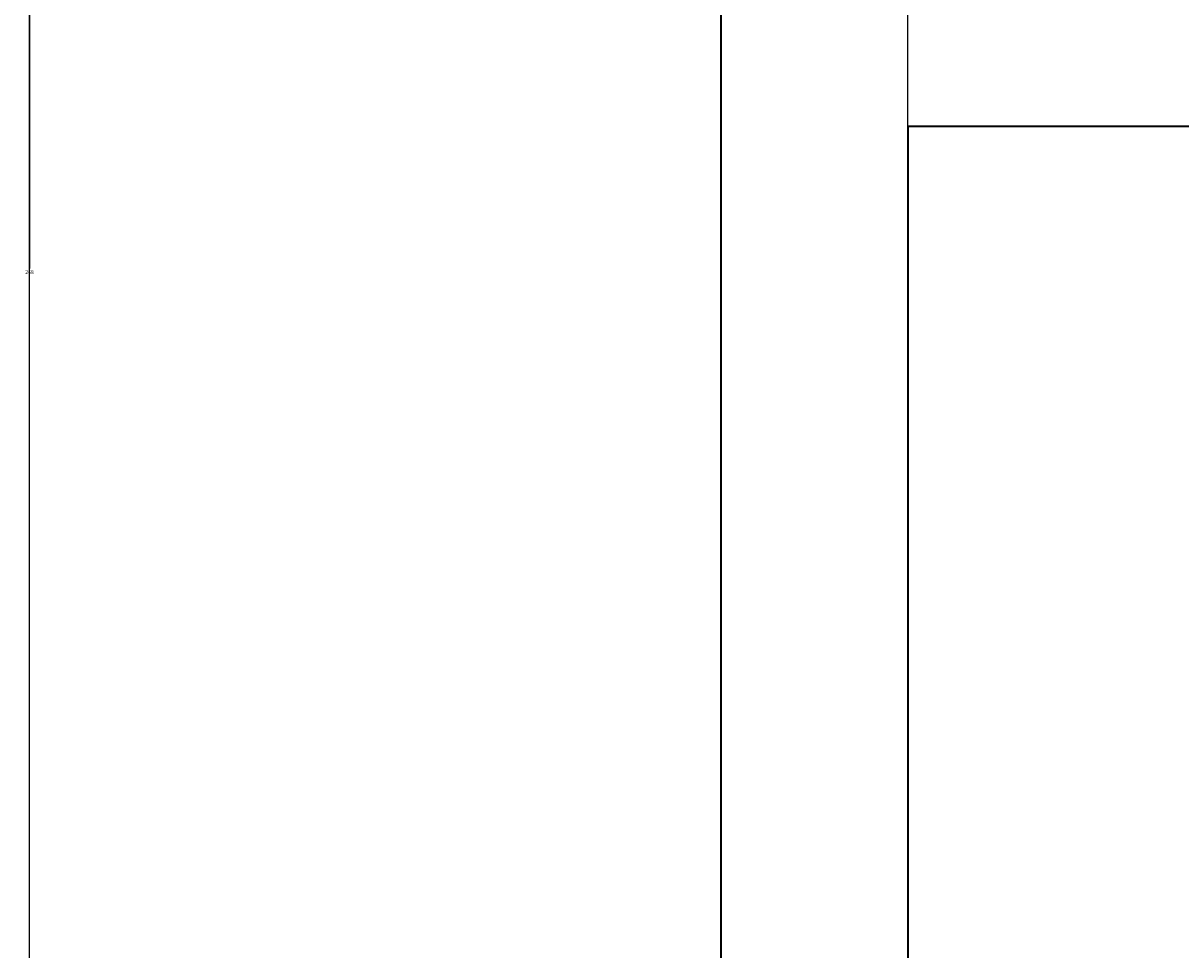
# Model space of a CAD drawing. Units: inches. Extents: x 4159 to 4826, y 299 to 1026.
# Tile 9 of 37: x 4159 to 4214, y 494 to 538. Entities that reach past the tile are written whole.
import ezdxf

# ---------------------------------------------------------------- set-up
doc = ezdxf.new("R2010")
doc.units = ezdxf.units.IN
doc.layers.add('A-ANNO-DIMS', color=2, linetype='Continuous', lineweight=18)
doc.layers.add('A-WALL', color=7, linetype='Continuous', lineweight=35)
doc.styles.get("Standard").update_dxf_attribs({"font": 'arial.ttf'})
doc.dimstyles.get("Standard").update_dxf_attribs({"dimtxt": 0.18, "dimasz": 0.18, "dimexe": 0.18, "dimexo": 0.0625, "dimgap": 0.09, "dimtad": 0, "dimtih": 1, "dimtoh": 1, "dimdec": 4, "dimzin": 0, "dimdsep": 46, "dimtxsty": 'Standard', "dimcen": 0.09, "dimadec": 0, "dimazin": 0, "dimtfac": 1, "dimtdec": 4, "dimtofl": 0, "dimtmove": 0, "dimatfit": 3, "dimfxl": 1, "dimtolj": 1, "dimtzin": 0, "dimarcsym": 0})

# ---------------------------------------------------------------- blocks, each defined once
blk = doc.blocks.new('*D44')
at = {"layer": 'A-ANNO-DIMS', "color": 0, "lineweight": -2, "transparency": 16777216}
for p, q in [((4287.263, 963.093), (4158.88, 963.093)), ((4159.06, 962.913), (4159.06, 647.826)), ((4159.06, 332.375), (4159.06, 647.462)), ((4447.248, 332.195), (4158.88, 332.195))]:
    blk.add_line(p, q, dxfattribs=at)
at = {"layer": 'A-ANNO-DIMS', "color": 0, "transparency": 16777216}
for points in [[(4159.03, 962.913), (4159.09, 962.913), (4159.06, 963.093)], [(4159.03, 332.375), (4159.09, 332.375), (4159.06, 332.195)]]:
    blk.add_solid(points, dxfattribs=at)
at = {"layer": 'Defpoints', "color": 0, "transparency": 16777216}
for p in [(4287.326, 963.093), (4159.06, 332.195), (4447.31, 332.195)]:
    blk.add_point(p, dxfattribs=at)
at = {"layer": 'A-ANNO-DIMS', "color": 0, "transparency": 16777216, "insert": (4159.06, 647.644), "char_height": 0.18, "attachment_point": 5}
blk.add_mtext('\\A1;630.9', dxfattribs=at)
blk = doc.blocks.new('*D50')
at = {"layer": 'A-ANNO-DIMS', "color": 0, "lineweight": -2, "transparency": 16777216}
for p, q in [((4192.31, 392.317), (4192.31, 1025.842)), ((4201.31, 401.317), (4201.31, 1025.842)), ((4192.49, 1025.662), (4196.661, 1025.662)), ((4201.13, 1025.662), (4196.959, 1025.662))]:
    blk.add_line(p, q, dxfattribs=at)
at = {"layer": 'A-ANNO-DIMS', "color": 0, "transparency": 16777216}
for points in [[(4192.49, 1025.692), (4192.49, 1025.632), (4192.31, 1025.662)], [(4201.13, 1025.692), (4201.13, 1025.632), (4201.31, 1025.662)]]:
    blk.add_solid(points, dxfattribs=at)
at = {"layer": 'Defpoints', "color": 0, "transparency": 16777216}
for p in [(4201.31, 1025.662), (4201.31, 401.254), (4192.31, 392.254)]:
    blk.add_point(p, dxfattribs=at)
at = {"layer": 'A-ANNO-DIMS', "color": 0, "transparency": 16777216, "insert": (4196.81, 1025.662), "char_height": 0.18, "attachment_point": 5}
blk.add_mtext('\\A1;9', dxfattribs=at)
blk = doc.blocks.new('*D51')
at = {"layer": 'A-ANNO-DIMS', "color": 0, "lineweight": -2, "transparency": 16777216}
for p, q in [((4201.248, 660.254), (4158.88, 660.254)), ((4159.06, 660.074), (4159.06, 526.436)), ((4159.06, 392.434), (4159.06, 526.072)), ((4192.248, 392.254), (4158.88, 392.254))]:
    blk.add_line(p, q, dxfattribs=at)
at = {"layer": 'A-ANNO-DIMS', "color": 0, "transparency": 16777216}
for points in [[(4159.03, 660.074), (4159.09, 660.074), (4159.06, 660.254)], [(4159.03, 392.434), (4159.09, 392.434), (4159.06, 392.254)]]:
    blk.add_solid(points, dxfattribs=at)
at = {"layer": 'Defpoints', "color": 0, "transparency": 16777216}
for p in [(4159.06, 660.254), (4201.31, 660.254), (4192.31, 392.254)]:
    blk.add_point(p, dxfattribs=at)
at = {"layer": 'A-ANNO-DIMS', "color": 0, "transparency": 16777216, "insert": (4159.06, 526.254), "char_height": 0.18, "attachment_point": 5}
blk.add_mtext('\\A1;268', dxfattribs=at)

msp = doc.modelspace()

# ---------------------------------------------------------------- linework, layer by layer
at = {"layer": 'A-WALL'}
for p, q in [((4201.31, 533.254), (4201.31, 401.254)), ((4279.31, 533.254), (4201.31, 533.254))]:
    msp.add_line(p, q, dxfattribs=at)
msp.add_lwpolyline([(4303.31, 903.254), (4192.31, 903.254), (4192.31, 392.254)], dxfattribs=at)

# ---------------------------------------------------------------- dimensions: what is measured, and where the dimension line sits
at = {"layer": 'A-ANNO-DIMS'}
dim = msp.add_linear_dim(base=(4201.31, 1025.662), p1=(4192.31, 392.254), p2=(4201.31, 401.254), dimstyle='Standard', override={"dimdec": 0, "dimlfac": 1, "dimrnd": 0, "dimzin": 0, "dimdsep": 46, "dimlunit": 2}, dxfattribs=at)
dim.commit()
dim.dimension.update_dxf_attribs({"geometry": '*D50', "text_midpoint": (4196.81, 1025.662)})
for base, p1, p2, override, picture, middle in [((4159.06, 332.195), (4287.326, 963.093), (4447.31, 332.195), {"dimdec": 1, "dimlfac": 1, "dimrnd": 0, "dimzin": 0, "dimdsep": 46, "dimlunit": 2}, '*D44', (4159.06, 647.644)), ((4159.06, 660.254), (4192.31, 392.254), (4201.31, 660.254), {"dimdec": 0, "dimlfac": 1, "dimrnd": 0, "dimzin": 0, "dimdsep": 46, "dimlunit": 2}, '*D51', (4159.06, 526.254))]:
    dim = msp.add_linear_dim(base=base, p1=p1, p2=p2, angle=90, dimstyle='Standard', override=override, dxfattribs=at)
    dim.commit()
    dim.dimension.update_dxf_attribs({"geometry": picture, "text_midpoint": middle})

doc.saveas('drawing.dxf')
